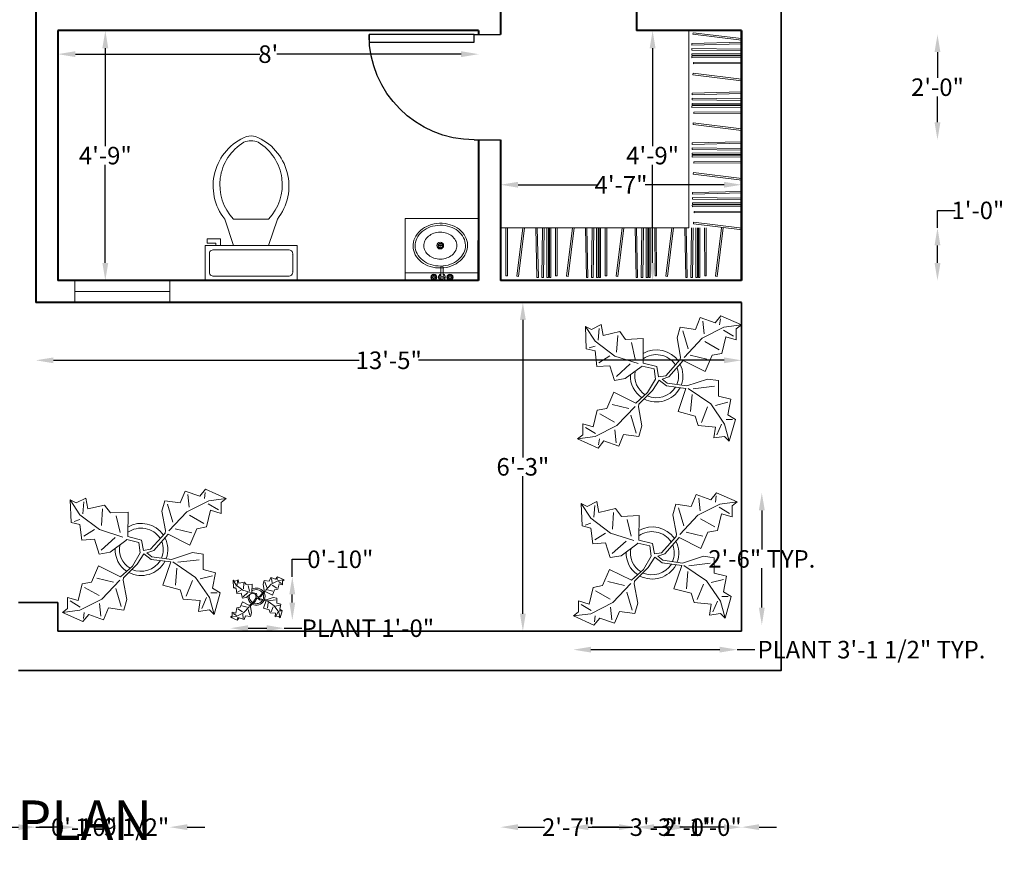
# Model space of a CAD drawing. Units: inches. Extents: x -46 to 447, y -42 to 702.
# Tile 2 of 7: x 222 to 447, y -42 to 148. Entities that reach past the tile are written whole.
import ezdxf

# ---------------------------------------------------------------- set-up
doc = ezdxf.new("R2010")
doc.units = ezdxf.units.IN
doc.header["$PDMODE"] = 3
for name, color, linetype, lineweight in [('A-ANNO-DIMS', 2, 'Continuous', 13), ('A-ANNO-TEXT', 3, 'Continuous', 25), ('A-DOOR', 3, 'Continuous', 25), ('A-FLOR-CASE', 32, 'Continuous', 18), ('A-FLOR-FIXT', 9, 'Continuous', 20), ('A-GLAZ', 4, 'Continuous', 18), ('A-WALL', 7, 'Continuous', 40), ('L-PLNT', 94, 'Continuous', 18), ('L-WALL', 7, 'Continuous', 35)]:
    doc.layers.add(name, color=color, linetype=linetype, lineweight=lineweight)
doc.styles.get("Standard").update_dxf_attribs({"font": 'arial.ttf'})
doc.dimstyles.get("Standard").update_dxf_attribs({"dimtxt": 4, "dimasz": 4, "dimexe": 0.18, "dimexo": 0.0625, "dimgap": 0.09, "dimtad": 0, "dimtih": 1, "dimtoh": 1, "dimdec": 0, "dimzin": 0, "dimdsep": 46, "dimlunit": 3, "dimtxsty": 'Standard', "dimcen": 0.09, "dimse1": 1, "dimse2": 1, "dimadec": 0, "dimazin": 0, "dimtfac": 1, "dimtdec": 0, "dimtofl": 0, "dimtmove": 0, "dimatfit": 3, "dimfxl": 1, "dimtolj": 1, "dimtzin": 0, "dimarcsym": 0})

# ---------------------------------------------------------------- blocks, each defined once
blk = doc.blocks.new('*U4')
for p, q in [((0, 0), (0, -6)), ((24, 0), (24, -6))]:
    blk.add_line(p, q)
blk.add_lwpolyline([(0, 0), (0, 24), (1.75, 24), (1.75, 0)], close=True)
blk.add_arc((0, 0), 24, 0, 90)
blk = doc.blocks.new('Plant - Rubber or Philodendron')
for p, q in [((8.8871, 10.7908), (9.9809, 13.4933)), ((9.9809, 13.4933), (13.3837, 12.301)), ((13.3837, 12.301), (14.68, 13.9039)), ((14.68, 13.9039), (19.3848, 11.8146)), ((-16.2005, 11.4774), (-13.9899, 8.1064)), ((-16.2005, 11.4774), (-14.8639, 10.7964)), ((-16.0159, 6.3329), (-16.2005, 11.4774)), ((-14.8639, 10.7964), (-12.6195, 11.8975)), ((-12.6195, 11.8975), (-12.1909, 9.4345)), ((4.6914, 8.8812), (5.3859, 11.2828)), ((5.3859, 11.2828), (8.8871, 10.7908)), ((15.3859, 11.3055), (10.3916, 8.7942)), ((10.5828, 12.6946), (10.8893, 9.7953)), ((14.5816, 13.2037), (14.3848, 11.8033)), ((19.3848, 11.8146), (15.3859, 11.3055)), ((19.3848, 11.8146), (18.1868, 10.9119)), ((-13.3174, 8.325), (-13.0735, 11.0065)), ((-12.1909, 9.4345), (-8.3829, 10.3)), ((-8.8369, 9.409), (-9.0894, 5.6095)), ((-8.3829, 10.3), (-7.0549, 8.501)), ((5.9878, 10.4842), (7.1971, 6.3869)), ((15.7909, 9.1065), (14.8995, 5.3044)), ((15.2875, 10.6053), (17.5907, 9.2105)), ((18.1925, 8.4119), (15.7909, 9.1065)), ((18.1868, 10.9119), (18.1925, 8.4119)), ((-15.3434, 6.5514), (-13.9984, 6.9884)), ((-13.9899, 8.1064), (-9.5434, 4.7185)), ((-7.0549, 8.501), (-3.0284, 8.6941)), ((-4.8529, 4.012), (-5.7184, 7.82)), ((-3.0284, 8.6941), (-3.0709, 3.1041)), ((4.6914, 8.8812), (5.5014, 4.4831)), ((10.3916, 8.7942), (6.2847, 4.4028)), ((14.2977, 6.1031), (10.9934, 7.9956)), ((-14.0069, 5.8704), (-16.0159, 6.3329)), ((-13.5868, 2.2894), (-14.0069, 5.8704)), ((-13.1329, 3.1804), (-10.6614, 4.727)), ((-9.5434, 4.7185), (-4.1917, 2.9888)), ((7.7005, 4.8881), (11.5025, 3.9967)), ((12.7005, 4.8994), (11.1089, 1.1958)), ((14.8995, 5.3044), (12.7005, 4.8994)), ((-10.6784, 2.491), (-13.5868, 2.2894)), ((-9.5858, -0.8715), (-10.6784, 2.491)), ((-9.1318, 0.0195), (-5.9793, 2.9025)), ((-3.5248, 2.2131), (-3.3011, 2.4355)), ((-3.3011, 2.4355), (-0.5306, 1.7947)), ((-3.0709, 3.1041), (0.0797, 2.3163)), ((0.0797, 2.3163), (0.4866, -0.031)), ((2.1141, 0.2298), (5.4346, 3.9146)), ((6.1032, 3.6844), (2.8262, -0.031)), ((5.4346, 3.9146), (5.5014, 4.4831)), ((11.1089, 1.1958), (6.1032, 3.6844)), ((-7.1228, -0.443), (-3.5248, 2.2131)), ((-0.5306, 1.7947), (-0.2255, -0.5527)), ((-0.5306, 1.7947), (-0.5306, 1.7947)), ((0.4866, -0.031), (2.1141, 0.2298)), ((-7.1228, -0.443), (-9.5858, -0.8715)), ((-2.019, -3.6148), (-0.2255, -0.5527)), ((-0.9375, -3.1608), (0.5883, -0.8135)), ((0.5883, -0.8135), (2.2447, -2.0916)), ((2.8262, -0.031), (1.3003, -0.5527)), ((1.3003, -0.5527), (2.4193, -1.4655)), ((2.2447, -2.0916), (6.7108, -2.6626)), ((2.4193, -1.4655), (6.895, -2.1175)), ((11.6605, -0.5413), (6.895, -2.1175)), ((8.3544, -2.7453), (13.1973, -2.1704)), ((11.6605, -0.5413), (14.1354, -0.8948)), ((14.1354, -0.8948), (14.1354, -4.4304)), ((-11.3237, -7.2629), (-9.7321, -3.5593)), ((-9.7321, -3.5593), (-4.7264, -6.0479)), ((-2.019, -3.6148), (-4.7264, -6.0479)), ((-4.0579, -6.2781), (-0.9375, -3.1608)), ((4.943, -7.9659), (6.7108, -2.6626)), ((12.3677, -6.1981), (7.219, -2.6772)), ((8.125, -4.0768), (7.7715, -7.9659)), ((14.1354, -4.4304), (16.9638, -5.1375)), ((-6.3237, -7.2516), (-10.1257, -6.3602)), ((-4.1246, -6.8466), (-4.0579, -6.2781)), ((15.5496, -10.7943), (12.3677, -6.1981)), ((16.2567, -5.8446), (13.4283, -6.5517)), ((16.9638, -5.1375), (16.2567, -8.673)), ((-14.4141, -11.4699), (-13.5228, -7.6679)), ((-13.5228, -7.6679), (-11.3237, -7.2629)), ((-12.921, -8.4665), (-9.6166, -10.359)), ((-9.0148, -11.1577), (-4.9047, -6.8122)), ((-4.611, -12.8477), (-5.8203, -8.7504)), ((-3.3146, -11.2447), (-4.1246, -6.8466)), ((8.8321, -9.0266), (4.943, -7.9659)), ((10.2463, -10.4408), (11.6605, -6.9053)), ((16.2567, -8.673), (18.0245, -9.7337)), ((-16.8157, -10.7754), (-14.4141, -11.4699)), ((-16.8101, -13.2754), (-16.8157, -10.7754)), ((-14.0091, -13.669), (-9.0148, -11.1577)), ((9.5392, -11.1479), (8.8321, -9.0266)), ((13.4283, -11.5015), (9.5392, -11.1479)), ((14.8425, -10.7943), (13.7819, -13.2692)), ((16.6103, -14.6834), (15.5496, -10.7943)), ((17.3174, -9.7337), (15.9032, -9.7337)), ((18.0245, -9.7337), (16.6103, -14.6834)), ((-18.008, -14.1781), (-16.8101, -13.2754)), ((-13.9107, -12.9688), (-16.2139, -11.574)), ((-9.206, -15.0581), (-9.5126, -12.1588)), ((-7.5103, -13.1543), (-8.6042, -15.8568)), ((-4.0092, -13.6463), (-7.5103, -13.1543)), ((-3.3146, -11.2447), (-4.0092, -13.6463)), ((13.0748, -13.9763), (13.4283, -11.5015)), ((-18.008, -14.1781), (-14.0091, -13.669)), ((-13.3032, -16.2674), (-18.008, -14.1781)), ((-12.0069, -14.6645), (-13.3032, -16.2674)), ((-13.2048, -15.5672), (-13.008, -14.1668)), ((-8.6042, -15.8568), (-12.0069, -14.6645)), ((15.5496, -13.6228), (13.0748, -13.9763)), ((16.6103, -14.6834), (15.5496, -13.6228))]:
    blk.add_line(p, q)
for centre, radius, start, end in [((0, 0), 6.1275, 34.37569, 120.1028), ((-0.0601, -0.2075), 5.2461, 33.82192, 124.9414), ((-0.098, 0.1364), 6.1288, 341.2017, 26.09184), ((0.0308, 0.1664), 6, 178.6147, 235.1169), ((0.0308, 0.1664), 5, 168.1647, 238.6725), ((-0.2664, 0.1682), 5.2775, 338.4094, 20.03007), ((-0.0234, 0.3825), 6.1492, 242.5812, 331.2714), ((-0.1102, 0.4886), 5.2883, 247.3711, 327.472)]:
    blk.add_arc(centre, radius, start, end)
blk = doc.blocks.new('Toilet - top')
for p, q in [((9.5, -6), (9.5, -2)), ((-10, -8.5), (-8, -8.5)), ((-10, -9.5), (-10, -8.5)), ((-8, -8.5), (-8, -8)), ((-7, -8), (-7, -9.5)), ((-4, -8), (-6, -14)), ((4, -8), (6, -14)), ((-7, -9.5), (-10, -9.5)), ((4, -14), (-4, -14))]:
    blk.add_line(p, q)
blk.add_lwpolyline([(10.5, -8), (10.5, 0), (-10.5, 0), (-10.5, -8)], close=True)
for points in [[(-9.5, -2), (-9.5, -6)], [(8.5, -1), (-8.5, -1)], [(-8.5, -7), (8.5, -7)]]:
    blk.add_lwpolyline(points)
for centre, radius, start, end in [((-8.62, -1.88), 0.884, 81.8699, 188.1301), ((8.62, -1.88), 0.884, 351.8699, 98.1301), ((-8.62, -6.12), 0.884, 171.8699, 278.1301), ((8.62, -6.12), 0.884, 261.8699, 8.1301), ((3.52, -21.58), 12.17, 141.4691, 247.9714), ((4.2, -21.82), 11.33, 136.3677, 238.9468), ((-3.52, -21.58), 12.17, 292.0284, 38.5307), ((-4.2, -21.82), 11.33, 301.053, 43.6321), ((0, -27.88), 4, 245.7318, 294.2682), ((0, -29), 4, 254.8605, 285.1395)]:
    blk.add_arc(centre, radius, start, end)
blk = doc.blocks.new('Faucet - Bathroom top')
for p, q in [((-4.107, 0.125), (-4.375, 0.125)), ((-3.75, 0.4788), (-3.75, 0.75)), ((-3.5, 0.482), (-3.5, 0.75)), ((-3.1461, 0.125), (-2.875, 0.125)), ((3.143, 0.125), (2.875, 0.125)), ((3.5, 0.4788), (3.5, 0.75)), ((3.75, 0.482), (3.75, 0.75)), ((4.1039, 0.125), (4.375, 0.125)), ((-4.1039, -0.125), (-4.375, -0.125)), ((-3.75, -0.4821), (-3.75, -0.75)), ((-3.5, -0.4789), (-3.5, -0.75)), ((-3.143, -0.125), (-2.875, -0.125)), ((-0.5, -0.8639), (-0.5, -4.5)), ((0.5, -4.5), (0.5, -0.8631)), ((3.1461, -0.125), (2.875, -0.125)), ((3.5, -0.4821), (3.5, -0.75)), ((3.75, -0.4789), (3.75, -0.75)), ((4.107, -0.125), (4.375, -0.125))]:
    blk.add_line(p, q)
for centre, radius in [((-3.625, 0), 1.375), ((-4.625, 0), 0.2795), ((-3.625, 0), 0.5), ((-3.625, 1), 0.2795), ((-2.625, 0), 0.2795), ((0, 0), 0.5), ((3.625, 0), 1.375), ((2.625, 0), 0.2795), ((3.625, 0), 0.5), ((3.625, 1), 0.2795), ((4.625, 0), 0.2795), ((-3.625, -1), 0.2795), ((3.625, -1), 0.2795)]:
    blk.add_circle(centre, radius)
for centre, radius, start, end in [((-3.625, 0), 1, 105.2407, 164.2093), ((-3.625, 0), 1, 16.44125, 74.07887), ((0, 0), 1.5, 289.6514, 250.3603), ((0, 0), 1, 300.3431, 239.7554), ((3.625, 0), 1, 106.12, 164.0884), ((3.625, 0), 1, 16.23422, 73.90469), ((-3.625, 0), 1, 196.2342, 253.9047), ((-3.625, 0), 1, 286.12, 344.0884), ((3.625, 0), 1, 196.4413, 254.0789), ((3.625, 0), 1, 285.2407, 344.2093), ((0, -4.5), 0.5, 180, 0)]:
    blk.add_arc(centre, radius, start, end)
blk = doc.blocks.new('Sink - Oval top')
for p, q in [((-1, 0), (1, 0)), ((0, 1), (0, -1))]:
    blk.add_line(p, q)
for points in [[(-12.23, 0.39, 0.117634), (-11.46, -3.36, 0.104469), (-8.88, -6.8, 0.090016), (-5.08, -9.07, 0.08192), (-0.32, -10.02, 0.08192), (4.49, -9.38, 0.090016), (8.42, -7.36, 0.104469), (11.22, -4.09, 0.117634), (12.23, -0.39, 0.117634), (11.46, 3.36, 0.104469), (8.88, 6.8, 0.090016), (5.08, 9.07, 0.08192), (0.32, 10.02, 0.08192), (-4.49, 9.38, 0.090016), (-8.42, 7.36, 0.104469), (-11.22, 4.09, 0.117634)], [(-11.29, 0.16, 0.118622), (-10.52, -3.25, 0.104678), (-8.07, -6.36, 0.089562), (-4.54, -8.37, 0.081185), (-0.13, -9.15, 0.081185), (4.3, -8.49, 0.089562), (7.89, -6.58, 0.104678), (10.42, -3.55, 0.118622), (11.29, -0.16, 0.118622), (10.52, 3.25, 0.104678), (8.07, 6.36, 0.089562), (4.54, 8.37, 0.081185), (0.13, 9.15, 0.081185), (-4.3, 8.49, 0.089562), (-7.89, 6.58, 0.104678), (-10.42, 3.55, 0.118622)], [(-7.42, 0.08, 0.118283), (-6.91, -2.17, 0.104607), (-5.29, -4.21, 0.089718), (-2.97, -5.53, 0.081436), (-0.07, -6.04, 0.081436), (2.84, -5.59, 0.089718), (5.2, -4.33, 0.104607), (6.86, -2.32, 0.118283), (7.42, -0.08, 0.118283), (6.91, 2.17, 0.104607), (5.29, 4.21, 0.089718), (2.97, 5.53, 0.081436), (0.07, 6.04, 0.081436), (-2.84, 5.59, 0.089718), (-5.2, 4.33, 0.104607), (-6.86, 2.32, 0.118283)]]:
    blk.add_lwpolyline(points, format="xyb", close=True)
for radius in [1.5, 1]:
    blk.add_circle((0, 0), radius)
blk = doc.blocks.new('*D53')
at = {"layer": 'A-ANNO-DIMS', "color": 0, "lineweight": -2, "transparency": 16777216}
for p, q in [((337.1, 80), (337.1, 48.63)), ((337.1, 13), (337.1, 44.37))]:
    blk.add_line(p, q, dxfattribs=at)
at = {"layer": 'A-ANNO-DIMS', "color": 0, "transparency": 16777216}
for points in [[(336.44, 80), (337.77, 80), (337.1, 84)], [(336.44, 13), (337.77, 13), (337.1, 9)]]:
    blk.add_solid(points, dxfattribs=at)
at = {"layer": 'Defpoints', "color": 0, "transparency": 16777216}
for p in [(337.1, 84), (387, 84), (387, 9)]:
    blk.add_point(p, dxfattribs=at)
at = {"layer": 'A-ANNO-DIMS', "color": 0, "transparency": 16777216, "insert": (337.1, 46.5), "char_height": 4, "attachment_point": 5}
blk.add_mtext('\\A1;6\'-3"', dxfattribs=at)
blk = doc.blocks.new('*D54')
at = {"layer": 'A-ANNO-DIMS', "color": 0, "lineweight": -2, "transparency": 16777216}
for p, q in [((230, 70.8), (299.73, 70.8)), ((383, 70.8), (313.27, 70.8))]:
    blk.add_line(p, q, dxfattribs=at)
at = {"layer": 'A-ANNO-DIMS', "color": 0, "transparency": 16777216}
for points in [[(230, 71.46), (230, 70.13), (226, 70.8)], [(383, 71.46), (383, 70.13), (387, 70.8)]]:
    blk.add_solid(points, dxfattribs=at)
at = {"layer": 'Defpoints', "color": 0, "transparency": 16777216}
for p in [(226, 84), (387, 84), (226, 70.8)]:
    blk.add_point(p, dxfattribs=at)
at = {"layer": 'A-ANNO-DIMS', "color": 0, "transparency": 16777216, "insert": (306.5, 70.8), "char_height": 4, "attachment_point": 5}
blk.add_mtext('\\A1;13\'-5"', dxfattribs=at)
blk = doc.blocks.new('*D55')
at = {"layer": 'A-ANNO-DIMS', "color": 0, "lineweight": -2, "transparency": 16777216}
for p, q in [((235, 140.64), (277.07, 140.64)), ((323, 140.64), (280.93, 140.64))]:
    blk.add_line(p, q, dxfattribs=at)
at = {"layer": 'A-ANNO-DIMS', "color": 0, "transparency": 16777216}
for points in [[(235, 141.31), (235, 139.97), (231, 140.64)], [(323, 141.31), (323, 139.97), (327, 140.64)]]:
    blk.add_solid(points, dxfattribs=at)
at = {"layer": 'Defpoints', "color": 0, "transparency": 16777216}
for p in [(231, 146), (327, 146), (231, 140.64)]:
    blk.add_point(p, dxfattribs=at)
at = {"layer": 'A-ANNO-DIMS', "color": 0, "transparency": 16777216, "insert": (279, 140.64), "char_height": 4, "attachment_point": 5}
blk.add_mtext("\\A1;8'", dxfattribs=at)
blk = doc.blocks.new('*D56')
at = {"layer": 'A-ANNO-DIMS', "color": 0, "lineweight": -2, "transparency": 16777216}
for p, q in [((241.83, 142), (241.83, 119.63)), ((241.83, 93), (241.83, 115.37))]:
    blk.add_line(p, q, dxfattribs=at)
at = {"layer": 'A-ANNO-DIMS', "color": 0, "transparency": 16777216}
for points in [[(241.16, 142), (242.5, 142), (241.83, 146)], [(241.16, 93), (242.5, 93), (241.83, 89)]]:
    blk.add_solid(points, dxfattribs=at)
at = {"layer": 'Defpoints', "color": 0, "transparency": 16777216}
for p in [(231, 146), (231, 89), (241.83, 89)]:
    blk.add_point(p, dxfattribs=at)
at = {"layer": 'A-ANNO-DIMS', "color": 0, "transparency": 16777216, "insert": (241.83, 117.5), "char_height": 4, "attachment_point": 5}
blk.add_mtext('\\A1;4\'-9"', dxfattribs=at)
blk = doc.blocks.new('*D57')
at = {"layer": 'A-ANNO-DIMS', "color": 0, "lineweight": -2, "transparency": 16777216}
for p, q in [((336, 110.85), (354.01, 110.85)), ((383, 110.85), (364.99, 110.85))]:
    blk.add_line(p, q, dxfattribs=at)
at = {"layer": 'A-ANNO-DIMS', "color": 0, "transparency": 16777216}
for points in [[(336, 111.51), (336, 110.18), (332, 110.85)], [(383, 111.51), (383, 110.18), (387, 110.85)]]:
    blk.add_solid(points, dxfattribs=at)
at = {"layer": 'Defpoints', "color": 0, "transparency": 16777216}
for p in [(332, 110.85), (332, 89), (387, 89)]:
    blk.add_point(p, dxfattribs=at)
at = {"layer": 'A-ANNO-DIMS', "color": 0, "transparency": 16777216, "insert": (359.5, 110.85), "char_height": 4, "attachment_point": 5}
blk.add_mtext('\\A1;4\'-7"', dxfattribs=at)
blk = doc.blocks.new('*D58')
at = {"layer": 'A-ANNO-DIMS', "color": 0, "lineweight": -2, "transparency": 16777216}
for p, q in [((366.7, 142), (366.7, 119.63)), ((366.7, 93), (366.7, 115.37))]:
    blk.add_line(p, q, dxfattribs=at)
at = {"layer": 'A-ANNO-DIMS', "color": 0, "transparency": 16777216}
for points in [[(366.04, 142), (367.37, 142), (366.7, 146)], [(366.04, 93), (367.37, 93), (366.7, 89)]]:
    blk.add_solid(points, dxfattribs=at)
at = {"layer": 'Defpoints', "color": 0, "transparency": 16777216}
for p in [(387, 146), (366.7, 89), (387, 89)]:
    blk.add_point(p, dxfattribs=at)
at = {"layer": 'A-ANNO-DIMS', "color": 0, "transparency": 16777216, "insert": (366.7, 117.5), "char_height": 4, "attachment_point": 5}
blk.add_mtext('\\A1;4\'-9"', dxfattribs=at)
blk = doc.blocks.new('VANITY-TOP')
for points in [[(0, -1.75), (16.74, -1.75), (16.74, 0), (0, 0)], [(0, -1.75), (16.74, -1.75), (16.74, -14.12), (0, -14.12)]]:
    blk.add_lwpolyline(points, close=True)
blk = doc.blocks.new('*D112')
at = {"layer": 'A-ANNO-DIMS', "color": 0, "lineweight": -2, "transparency": 16777216}
for p, q in [((352.62, 4.79), (382.01, 4.79)), ((386.01, 4.79), (390.01, 4.79))]:
    blk.add_line(p, q, dxfattribs=at)
at = {"layer": 'A-ANNO-DIMS', "color": 0, "transparency": 16777216}
for points in [[(352.62, 5.46), (352.62, 4.13), (348.62, 4.79)], [(382.01, 5.46), (382.01, 4.13), (386.01, 4.79)]]:
    blk.add_solid(points, dxfattribs=at)
at = {"layer": 'Defpoints', "color": 0, "transparency": 16777216}
for p in [(348.62, 10.4), (386.01, 10.4), (386.01, 4.79)]:
    blk.add_point(p, dxfattribs=at)
at = {"layer": 'A-ANNO-DIMS', "color": 0, "transparency": 16777216, "insert": (416.64, 4.79), "char_height": 4, "attachment_point": 5}
blk.add_mtext('\\A1;PLANT 3\'-1 1/2" TYP.', dxfattribs=at)
blk = doc.blocks.new('*D113')
at = {"layer": 'A-ANNO-DIMS', "color": 0, "lineweight": -2, "transparency": 16777216}
for p, q in [((391.62, 36.57), (391.62, 27.62)), ((391.62, 14.4), (391.62, 23.36))]:
    blk.add_line(p, q, dxfattribs=at)
at = {"layer": 'A-ANNO-DIMS', "color": 0, "transparency": 16777216}
for points in [[(390.95, 36.57), (392.29, 36.57), (391.62, 40.57)], [(390.95, 14.4), (392.29, 14.4), (391.62, 10.4)]]:
    blk.add_solid(points, dxfattribs=at)
at = {"layer": 'Defpoints', "color": 0, "transparency": 16777216}
for p in [(386.01, 40.57), (391.62, 40.57), (386.01, 10.4)]:
    blk.add_point(p, dxfattribs=at)
at = {"layer": 'A-ANNO-DIMS', "color": 0, "transparency": 16777216, "insert": (391.62, 25.49), "char_height": 4, "attachment_point": 5}
blk.add_mtext('\\A1;2\'-6" TYP.', dxfattribs=at)
blk = doc.blocks.new('*D114')
at = {"layer": 'A-ANNO-DIMS', "color": 0, "lineweight": -2, "transparency": 16777216}
for p, q in [((274.41, 9.69), (278.65, 9.69)), ((282.65, 9.69), (286.65, 9.69))]:
    blk.add_line(p, q, dxfattribs=at)
at = {"layer": 'A-ANNO-DIMS', "color": 0, "transparency": 16777216}
for points in [[(274.41, 10.36), (274.41, 9.02), (270.41, 9.69)], [(278.65, 10.36), (278.65, 9.02), (282.65, 9.69)]]:
    blk.add_solid(points, dxfattribs=at)
at = {"layer": 'Defpoints', "color": 0, "transparency": 16777216}
for p in [(270.41, 11.53), (282.65, 11.53), (282.65, 9.69)]:
    blk.add_point(p, dxfattribs=at)
at = {"layer": 'A-ANNO-DIMS', "color": 0, "transparency": 16777216, "insert": (301.74, 9.69), "char_height": 4, "attachment_point": 5}
blk.add_mtext('\\A1;PLANT 1\'-0"', dxfattribs=at)
blk = doc.blocks.new('*D115')
at = {"layer": 'A-ANNO-DIMS', "color": 0, "lineweight": -2, "transparency": 16777216}
for p, q in [((284.49, 21.41), (284.49, 25.41)), ((284.49, 25.41), (288.49, 25.41)), ((284.49, 15.53), (284.49, 17.41))]:
    blk.add_line(p, q, dxfattribs=at)
at = {"layer": 'A-ANNO-DIMS', "color": 0, "transparency": 16777216}
for points in [[(283.82, 17.41), (285.16, 17.41), (284.49, 21.41)], [(283.82, 15.53), (285.16, 15.53), (284.49, 11.53)]]:
    blk.add_solid(points, dxfattribs=at)
at = {"layer": 'Defpoints', "color": 0, "transparency": 16777216}
for p in [(282.65, 21.41), (284.49, 21.41), (282.65, 11.53)]:
    blk.add_point(p, dxfattribs=at)
at = {"layer": 'A-ANNO-DIMS', "color": 0, "transparency": 16777216, "insert": (295.45, 25.41), "char_height": 4, "attachment_point": 5}
blk.add_mtext('\\A1;0\'-10"', dxfattribs=at)
blk = doc.blocks.new('*D118')
at = {"layer": 'A-ANNO-DIMS', "color": 0, "lineweight": -2, "transparency": 16777216}
for p, q in [((352, -35.7), (362.09, -35.7)), ((383, -35.7), (372.91, -35.7))]:
    blk.add_line(p, q, dxfattribs=at)
at = {"layer": 'A-ANNO-DIMS', "color": 0, "transparency": 16777216}
for points in [[(352, -35.03), (352, -36.37), (348, -35.7)], [(383, -35.03), (383, -36.37), (387, -35.7)]]:
    blk.add_solid(points, dxfattribs=at)
at = {"layer": 'Defpoints', "color": 0, "transparency": 16777216}
for p in [(348, 324), (387, 324), (387, -35.7)]:
    blk.add_point(p, dxfattribs=at)
at = {"layer": 'A-ANNO-DIMS', "color": 0, "transparency": 16777216, "insert": (367.5, -35.7), "char_height": 4, "attachment_point": 5}
blk.add_mtext('\\A1;3\'-3"', dxfattribs=at)
blk = doc.blocks.new('*D120')
at = {"layer": 'A-ANNO-DIMS', "color": 0, "lineweight": -2, "transparency": 16777216}
for p, q in [((336, -35.7), (342.06, -35.7)), ((359, -35.7), (352.94, -35.7))]:
    blk.add_line(p, q, dxfattribs=at)
at = {"layer": 'A-ANNO-DIMS', "color": 0, "transparency": 16777216}
for points in [[(336, -35.03), (336, -36.37), (332, -35.7)], [(359, -35.03), (359, -36.37), (363, -35.7)]]:
    blk.add_solid(points, dxfattribs=at)
at = {"layer": 'Defpoints', "color": 0, "transparency": 16777216}
for p in [(332, 151), (363, 151), (363, -35.7)]:
    blk.add_point(p, dxfattribs=at)
at = {"layer": 'A-ANNO-DIMS', "color": 0, "transparency": 16777216, "insert": (347.5, -35.7), "char_height": 4, "attachment_point": 5}
blk.add_mtext('\\A1;2\'-7"', dxfattribs=at)
blk = doc.blocks.new('*D131')
at = {"layer": 'A-ANNO-DIMS', "color": 0, "lineweight": -2, "transparency": 16777216}
for p, q in [((431.7, 141.1), (431.7, 135.23)), ((431.7, 125.1), (431.7, 130.96))]:
    blk.add_line(p, q, dxfattribs=at)
at = {"layer": 'A-ANNO-DIMS', "color": 0, "transparency": 16777216}
for points in [[(431.03, 141.1), (432.37, 141.1), (431.7, 145.1)], [(431.03, 125.1), (432.37, 125.1), (431.7, 121.1)]]:
    blk.add_solid(points, dxfattribs=at)
at = {"layer": 'Defpoints', "color": 0, "transparency": 16777216}
for p in [(332, 145.1), (431.7, 145.1), (332, 121.1)]:
    blk.add_point(p, dxfattribs=at)
at = {"layer": 'A-ANNO-DIMS', "color": 0, "transparency": 16777216, "insert": (431.7, 133.1), "char_height": 4, "attachment_point": 5}
blk.add_mtext('\\A1;2\'-0"', dxfattribs=at)
blk = doc.blocks.new('*D132')
at = {"layer": 'A-ANNO-DIMS', "color": 0, "lineweight": -2, "transparency": 16777216}
for p, q in [((230.84, -35.7), (226.84, -35.7)), ((260.52, -35.7), (264.52, -35.7))]:
    blk.add_line(p, q, dxfattribs=at)
at = {"layer": 'A-ANNO-DIMS', "color": 0, "transparency": 16777216}
for points in [[(230.84, -35.03), (230.84, -36.37), (234.84, -35.7)], [(260.52, -35.03), (260.52, -36.37), (256.52, -35.7)]]:
    blk.add_solid(points, dxfattribs=at)
at = {"layer": 'Defpoints', "color": 0, "transparency": 16777216}
for p in [(234.84, 84), (256.52, 84), (256.52, -35.7)]:
    blk.add_point(p, dxfattribs=at)
at = {"layer": 'A-ANNO-DIMS', "color": 0, "transparency": 16777216, "insert": (245.68, -35.7), "char_height": 4, "attachment_point": 5}
blk.add_mtext('\\A1;1\'-9 1/2"', dxfattribs=at)
blk = doc.blocks.new('*D143')
at = {"layer": 'A-ANNO-DIMS', "color": 0, "lineweight": -2, "transparency": 16777216}
for p, q in [((220.17, -35.7), (222, -35.7)), ((226, -35.7), (230, -35.7))]:
    blk.add_line(p, q, dxfattribs=at)
at = {"layer": 'A-ANNO-DIMS', "color": 0, "transparency": 16777216}
for points in [[(220.17, -35.03), (220.17, -36.37), (216.17, -35.7)], [(222, -35.03), (222, -36.37), (226, -35.7)]]:
    blk.add_solid(points, dxfattribs=at)
at = {"layer": 'Defpoints', "color": 0, "transparency": 16777216}
for p in [(216.17, 201), (226, 201), (226, -35.7)]:
    blk.add_point(p, dxfattribs=at)
at = {"layer": 'A-ANNO-DIMS', "color": 0, "transparency": 16777216, "insert": (236.96, -35.7), "char_height": 4, "attachment_point": 5}
blk.add_mtext('\\A1;0\'-10"', dxfattribs=at)
blk = doc.blocks.new('*D147')
at = {"layer": 'A-ANNO-DIMS', "color": 0, "lineweight": -2, "transparency": 16777216}
for p, q in [((367, -35.7), (369.56, -35.7)), ((383, -35.7), (380.44, -35.7))]:
    blk.add_line(p, q, dxfattribs=at)
at = {"layer": 'A-ANNO-DIMS', "color": 0, "transparency": 16777216}
for points in [[(367, -35.03), (367, -36.37), (363, -35.7)], [(383, -35.03), (383, -36.37), (387, -35.7)]]:
    blk.add_solid(points, dxfattribs=at)
at = {"layer": 'Defpoints', "color": 0, "transparency": 16777216}
for p in [(363, 151), (387, 151), (387, -35.7)]:
    blk.add_point(p, dxfattribs=at)
at = {"layer": 'A-ANNO-DIMS', "color": 0, "transparency": 16777216, "insert": (375, -35.7), "char_height": 4, "attachment_point": 5}
blk.add_mtext('\\A1;2\'-0"', dxfattribs=at)
blk = doc.blocks.new('*D153')
at = {"layer": 'A-ANNO-DIMS', "color": 0, "lineweight": -2, "transparency": 16777216}
for p, q in [((371, -35.7), (367, -35.7)), ((391, -35.7), (395, -35.7))]:
    blk.add_line(p, q, dxfattribs=at)
at = {"layer": 'A-ANNO-DIMS', "color": 0, "transparency": 16777216}
for points in [[(371, -35.03), (371, -36.37), (375, -35.7)], [(391, -35.03), (391, -36.37), (387, -35.7)]]:
    blk.add_solid(points, dxfattribs=at)
at = {"layer": 'Defpoints', "color": 0, "transparency": 16777216}
for p in [(375, 146), (387, 146), (387, -35.7)]:
    blk.add_point(p, dxfattribs=at)
at = {"layer": 'A-ANNO-DIMS', "color": 0, "transparency": 16777216, "insert": (381, -35.7), "char_height": 4, "attachment_point": 5}
blk.add_mtext('\\A1;1\'-0"', dxfattribs=at)
blk = doc.blocks.new('*D154')
at = {"layer": 'A-ANNO-DIMS', "color": 0, "lineweight": -2, "transparency": 16777216}
for p, q in [((431.7, 101), (431.7, 105)), ((431.7, 105), (435.7, 105)), ((431.7, 93), (431.7, 97))]:
    blk.add_line(p, q, dxfattribs=at)
at = {"layer": 'A-ANNO-DIMS', "color": 0, "transparency": 16777216}
for points in [[(431.03, 97), (432.37, 97), (431.7, 101)], [(431.03, 93), (432.37, 93), (431.7, 89)]]:
    blk.add_solid(points, dxfattribs=at)
at = {"layer": 'Defpoints', "color": 0, "transparency": 16777216}
for p in [(332, 101), (431.7, 101), (332, 89)]:
    blk.add_point(p, dxfattribs=at)
at = {"layer": 'A-ANNO-DIMS', "color": 0, "transparency": 16777216, "insert": (440.92, 105), "char_height": 4, "attachment_point": 5}
blk.add_mtext('\\A1;1\'-0"', dxfattribs=at)

msp = doc.modelspace()

# ---------------------------------------------------------------- linework, layer by layer
at = {"layer": 'A-FLOR-CASE'}
for p, q in [((375, 146), (375, 101)), ((375, 101), (332, 101))]:
    msp.add_line(p, q, dxfattribs=at)
for points in [[(387, 144.2), (375.95, 145.53), (375.91, 145.18), (387, 143.84)], [(386.95, 142.99), (375.65, 142.71), (375.64, 143.06), (386.95, 143.34)], [(386.95, 141.42), (375.65, 141.55), (375.65, 141.9), (386.95, 141.77)], [(386.96, 139.88), (375.63, 139.83), (375.63, 140.18), (386.96, 140.23)], [(386.96, 140.44), (375.65, 140.39), (375.65, 140.74), (386.96, 140.79)], [(386.96, 138.49), (376.05, 138.4), (376.05, 138.76), (386.96, 138.84)], [(386.98, 134.94), (375.93, 136.27), (375.89, 135.93), (386.98, 134.58)], [(386.99, 131.66), (375.7, 131.38), (375.69, 131.73), (386.99, 132.01)], [(387, 130.09), (375.69, 130.22), (375.7, 130.57), (387, 130.44)], [(387, 128.54), (375.68, 128.5), (375.67, 128.85), (387, 128.9)], [(387, 129.11), (375.7, 129.06), (375.7, 129.41), (387, 129.46)], [(387.01, 127.16), (376.1, 127.07), (376.09, 127.42), (387.01, 127.51)], [(387.02, 123.61), (375.98, 124.94), (375.93, 124.59), (387.02, 123.25)], [(387.04, 120.32), (375.74, 120.05), (375.73, 120.4), (387.03, 120.67)], [(387.04, 118.75), (375.74, 118.89), (375.74, 119.24), (387.04, 119.11)], [(387.05, 117.21), (375.72, 117.17), (375.72, 117.52), (387.05, 117.56)], [(387.05, 117.77), (375.74, 117.73), (375.74, 118.08), (387.04, 118.13)], [(387.05, 115.83), (376.14, 115.74), (376.14, 116.09), (387.05, 116.18)], [(387.07, 112.28), (376.02, 113.61), (375.98, 113.26), (387.07, 111.92)], [(387.08, 108.99), (375.79, 108.71), (375.78, 109.07), (387.08, 109.34)], [(387.09, 107.42), (375.78, 107.55), (375.79, 107.91), (387.09, 107.77)], [(387.09, 105.88), (375.77, 105.84), (375.76, 106.19), (387.09, 106.23)], [(387.09, 106.44), (375.79, 106.4), (375.79, 106.75), (387.09, 106.79)], [(387.1, 104.5), (376.18, 104.41), (376.18, 104.76), (387.1, 104.85)], [(387.11, 100.94), (376.06, 102.28), (376.02, 101.93), (387.11, 100.59)], [(333.56, 101), (333.6, 90.09), (333.25, 90.08), (333.21, 101)], [(337.11, 101), (335.73, 89.96), (336.08, 89.91), (337.47, 101)], [(340.39, 101), (340.63, 89.7), (340.28, 89.7), (340.04, 101)], [(341.96, 101), (341.79, 89.7), (341.44, 89.7), (341.61, 101)], [(342.94, 101), (342.94, 89.7), (342.59, 89.7), (342.59, 101)], [(343.51, 101), (343.51, 89.67), (343.15, 89.67), (343.15, 101)], [(344.89, 101), (344.93, 90.09), (344.58, 90.08), (344.54, 101)], [(348.44, 101), (347.06, 89.96), (347.41, 89.91), (348.8, 101)], [(351.73, 101), (351.96, 89.7), (351.61, 89.7), (351.38, 101)], [(353.3, 101), (353.12, 89.7), (352.77, 89.7), (352.94, 101)], [(354.28, 101), (354.28, 89.7), (353.92, 89.7), (353.92, 101)], [(354.84, 101), (354.84, 89.67), (354.49, 89.67), (354.49, 101)], [(356.22, 101), (356.27, 90.09), (355.91, 90.08), (355.87, 101)], [(359.77, 101), (358.39, 89.96), (358.74, 89.91), (360.13, 101)], [(363.06, 101), (363.29, 89.7), (362.94, 89.7), (362.71, 101)], [(364.63, 101), (364.45, 89.7), (364.1, 89.7), (364.28, 101)], [(365.61, 101), (365.61, 89.7), (365.26, 89.7), (365.26, 101)], [(366.17, 101), (366.17, 89.67), (365.82, 89.67), (365.82, 101)], [(367.55, 101), (367.6, 90.09), (367.25, 90.08), (367.2, 101)], [(371.11, 101), (369.73, 89.96), (370.07, 89.91), (371.46, 101)], [(374.39, 101), (374.62, 89.7), (374.27, 89.7), (374.04, 101)], [(375.96, 101), (375.78, 89.7), (375.43, 89.7), (375.61, 101)], [(376.94, 101), (376.94, 89.7), (376.59, 89.7), (376.59, 101)], [(377.5, 101), (377.5, 89.67), (377.15, 89.67), (377.15, 101)], [(378.89, 101), (378.93, 90.09), (378.58, 90.08), (378.53, 101)], [(382.44, 101), (381.06, 89.96), (381.41, 89.91), (382.79, 101)]]:
    msp.add_lwpolyline(points, dxfattribs=at)
at = {"layer": 'A-GLAZ'}
for p, q in [((234.84, 89), (234.84, 84)), ((256.52, 89), (256.52, 84)), ((234.84, 86.5), (256.52, 86.5))]:
    msp.add_line(p, q, dxfattribs=at)
at = {"layer": 'A-WALL'}
for p, q in [((226, 201), (226, 84)), ((332, 151), (332, 145.1)), ((363, 151), (363, 146)), ((327, 146), (231, 146)), ((231, 146), (231, 89)), ((327, 146), (327, 145.1)), ((387, 146), (363, 146)), ((387, 146), (387, 89)), ((387, 89), (387, 146)), ((327, 121.1), (327, 89)), ((332, 121.1), (332, 89)), ((327, 89), (327, 98.15)), ((327, 89), (231, 89)), ((387, 89), (332, 89)), ((387, 84), (226, 84))]:
    msp.add_line(p, q, dxfattribs=at)
at = {"layer": 'L-WALL'}
for p, q in [((387, 9), (387, 84)), ((231, 15.54), (222, 15.54)), ((231, 15.54), (231, 9)), ((231, 9), (387, 9))]:
    msp.add_line(p, q, dxfattribs=at)
msp.add_lwpolyline([(222, 0), (396, 0), (396, 660), (0, 660), (0, 0), (17.93, 0)], dxfattribs=at)

# ---------------------------------------------------------------- block references
at = {"layer": 'A-DOOR', "xscale": -1, "rotation": 90}
msp.add_blockref('*U4', (326, 145.1), dxfattribs=at)
at = {"layer": 'A-FLOR-CASE', "extrusion": (0, 0, -1), "zscale": -1, "rotation": 180}
msp.add_blockref('VANITY-TOP', (-310.26, 89), dxfattribs=at)
at = {"layer": 'A-FLOR-FIXT', "xscale": -1, "rotation": 180}
msp.add_blockref('Toilet - top', (275.08, 89), dxfattribs=at)
at = {"layer": 'A-FLOR-FIXT', "xscale": -0.5085474315686545, "yscale": 0.5085474315686545, "zscale": 0.5085474315686545, "rotation": 180}
for name, p in [('Sink - Oval top', (318.26, 96.96)), ('Faucet - Bathroom top', (318.63, 89.76))]:
    msp.add_blockref(name, p, dxfattribs=at)
at = {"layer": 'L-PLNT'}
for p in [(367.59, 67.06), (250.04, 27.47), (366.63, 26.67)]:
    msp.add_blockref('Plant - Rubber or Philodendron', p, dxfattribs=at)
at = {"layer": 'L-PLNT', "xscale": 0.3274952468944182, "yscale": 0.3274952468944182, "zscale": 0.3274952468944182}
msp.add_blockref('Plant - Rubber or Philodendron', (276.3, 16.85), dxfattribs=at)

# ---------------------------------------------------------------- texts
at = {"layer": 'A-ANNO-TEXT', "insert": (125.24, -29.6), "char_height": 9, "attachment_point": 1}
msp.add_mtext_dynamic_manual_height_columns('GROUND FLOOR PLAN', width=170.7105, gutter_width=12.5, heights=[0], dxfattribs=at)

# ---------------------------------------------------------------- dimensions: what is measured, and where the dimension line sits
at = {"layer": 'A-ANNO-DIMS'}
for base, p1, p2, override, picture, middle in [((387, -35.7), (348, 324), (387, 324), {"dimdec": 1, "dimlfac": 1, "dimrnd": 0, "dimzin": 1, "dimdsep": 46, "dimlunit": 4, "dimfrac": 2}, '*D118', (367.5, -35.7)), ((226, -35.7), (216.17, 201), (226, 201), {"dimdec": 1, "dimlfac": 1, "dimrnd": 0, "dimzin": 1, "dimdsep": 46, "dimlunit": 4, "dimfrac": 2}, '*D143', (236.96, -35.7)), ((363, -35.7), (332, 151), (363, 151), {"dimdec": 1, "dimlfac": 1, "dimrnd": 0, "dimzin": 1, "dimdsep": 46, "dimlunit": 4, "dimfrac": 2}, '*D120', (347.5, -35.7)), ((387, -35.7), (363, 151), (387, 151), {"dimdec": 1, "dimlfac": 1, "dimrnd": 0, "dimzin": 1, "dimdsep": 46, "dimlunit": 4, "dimfrac": 2}, '*D147', (375, -35.7)), ((231, 140.64), (327, 146), (231, 146), {"dimclrd": 0, "dimclre": 0, "dimclrt": 0}, '*D55', (279, 140.64)), ((387, -35.7), (375, 146), (387, 146), {"dimdec": 1, "dimlfac": 1, "dimrnd": 0, "dimzin": 1, "dimdsep": 46, "dimlunit": 4, "dimfrac": 2}, '*D153', (381, -35.7)), ((332, 110.85), (387, 89), (332, 89), {"dimclrd": 0, "dimclre": 0, "dimclrt": 0}, '*D57', (359.5, 110.85)), ((226, 70.8), (387, 84), (226, 84), {"dimclrd": 0, "dimclre": 0, "dimclrt": 0}, '*D54', (306.5, 70.8)), ((256.52, -35.7), (234.84, 84), (256.52, 84), {"dimdec": 1, "dimlfac": 1, "dimrnd": 0, "dimzin": 1, "dimdsep": 46, "dimlunit": 4, "dimfrac": 2}, '*D132', (245.68, -35.7))]:
    dim = msp.add_linear_dim(base=base, p1=p1, p2=p2, dimstyle='Standard', override=override, dxfattribs=at)
    dim.commit()
    dim.dimension.update_dxf_attribs({"geometry": picture, "text_midpoint": middle})
for base, p1, p2, override, picture, middle in [((241.83, 89), (231, 146), (231, 89), {"dimclrd": 0, "dimclre": 0, "dimclrt": 0}, '*D56', (241.83, 117.5)), ((431.7, 145.1), (332, 121.1), (332, 145.1), {"dimdec": 1, "dimlfac": 1, "dimrnd": 0, "dimzin": 1, "dimdsep": 46, "dimlunit": 4, "dimfrac": 2}, '*D131', (431.7, 133.1)), ((366.7, 89), (387, 146), (387, 89), {"dimclrd": 0, "dimclre": 0, "dimclrt": 0}, '*D58', (366.7, 117.5)), ((431.7, 101), (332, 89), (332, 101), {"dimdec": 1, "dimlfac": 1, "dimrnd": 0, "dimzin": 1, "dimdsep": 46, "dimlunit": 4, "dimfrac": 2}, '*D154', (440.92, 105)), ((337.1, 84), (387, 9), (387, 84), {"dimclrd": 0, "dimclre": 0, "dimclrt": 0}, '*D53', (337.1, 46.5)), ((284.49, 21.41), (282.65, 11.53), (282.65, 21.41), {"dimdec": 1, "dimlfac": 1, "dimrnd": 0, "dimzin": 1, "dimdsep": 46, "dimlunit": 4, "dimfrac": 2}, '*D115', (295.45, 25.41))]:
    dim = msp.add_linear_dim(base=base, p1=p1, p2=p2, angle=90, dimstyle='Standard', override=override, dxfattribs=at)
    dim.commit()
    dim.dimension.update_dxf_attribs({"geometry": picture, "text_midpoint": middle})
dim = msp.add_linear_dim(base=(391.62, 40.57), p1=(386.01, 10.4), p2=(386.01, 40.57), angle=90, text='<> TYP.', dimstyle='Standard', override={"dimdec": 1, "dimlfac": 1, "dimrnd": 0, "dimzin": 1, "dimdsep": 46, "dimlunit": 4, "dimfrac": 2}, dxfattribs=at)
dim.commit()
dim.dimension.update_dxf_attribs({"geometry": '*D113', "text_midpoint": (391.62, 25.49)})
for base, p1, p2, text, picture, middle in [((386.01, 4.79), (348.62, 10.4), (386.01, 10.4), 'PLANT <> TYP.', '*D112', (416.64, 4.79)), ((282.65, 9.69), (270.41, 11.53), (282.65, 11.53), 'PLANT <>', '*D114', (301.74, 9.69))]:
    dim = msp.add_linear_dim(base=base, p1=p1, p2=p2, text=text, dimstyle='Standard', override={"dimdec": 1, "dimlfac": 1, "dimrnd": 0, "dimzin": 1, "dimdsep": 46, "dimlunit": 4, "dimfrac": 2}, dxfattribs=at)
    dim.commit()
    dim.dimension.update_dxf_attribs({"geometry": picture, "text_midpoint": middle})

doc.saveas('drawing.dxf')
